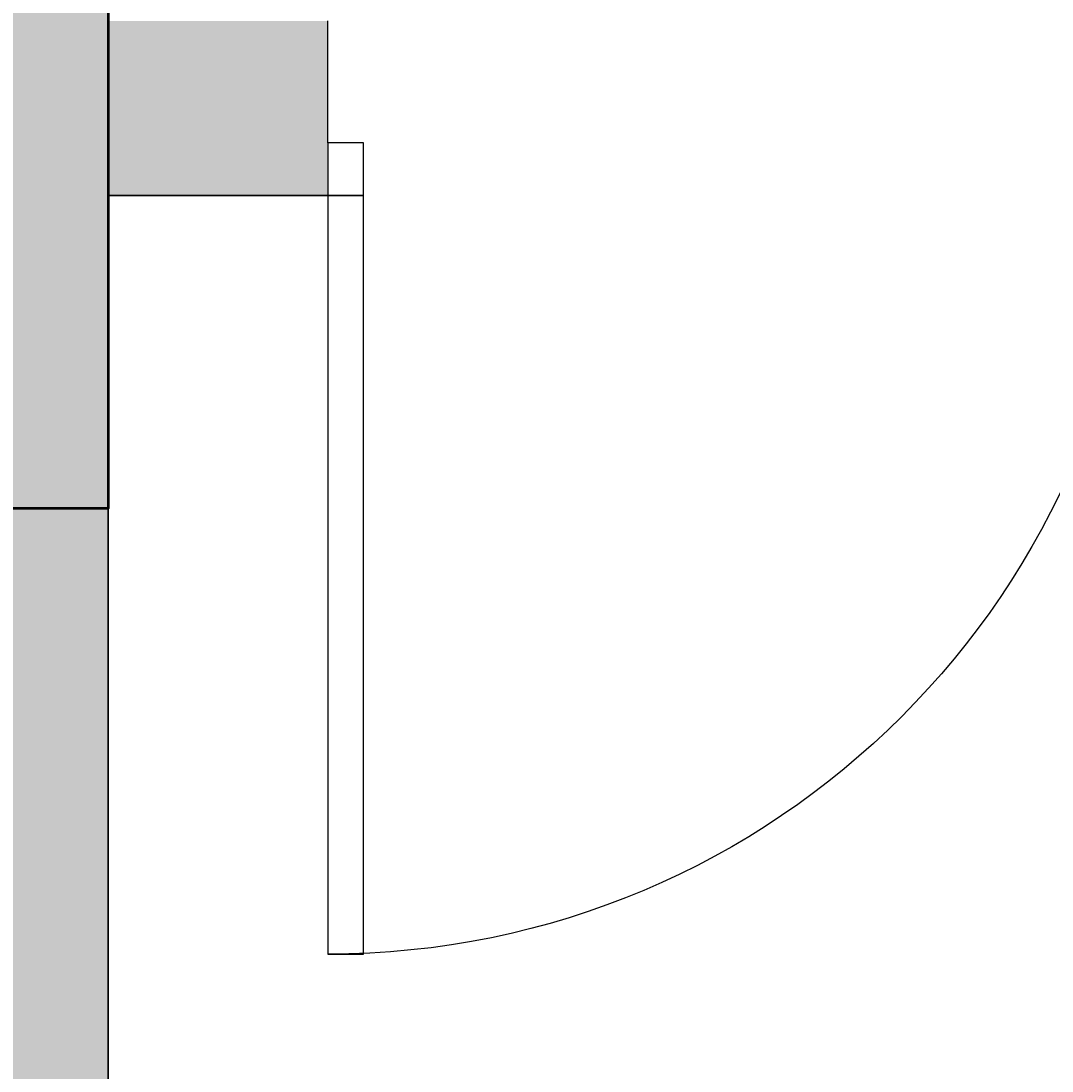
# Model space of a CAD drawing. Units: inches. Extents: x 1998 to 2588, y 1139 to 1977.
# Tile 78 of 134: x 2344 to 2370, y 1454 to 1481. Entities that reach past the tile are written whole.
import ezdxf

# ---------------------------------------------------------------- set-up
doc = ezdxf.new("R2010")
doc.units = ezdxf.units.IN
for name, color, linetype, lineweight in [('A-ANNO-DIMS', 2, 'Continuous', 18), ('A-COLS-PATT', 250, 'Continuous', 13), ('A-WALL-PATT', 252, 'Continuous', 13), ('COLUMN', 10, 'Continuous', 50), ('DOOR', 52, 'Continuous', 25), ('WALL', 200, 'Continuous', 35)]:
    doc.layers.add(name, color=color, linetype=linetype, lineweight=lineweight)
doc.styles.get("Standard").update_dxf_attribs({"font": 'arial.ttf'})
doc.dimstyles.get("Standard").update_dxf_attribs({"dimtxt": 0.18, "dimasz": 0.18, "dimexe": 0.18, "dimexo": 0.0625, "dimgap": 0.09, "dimtad": 0, "dimtih": 1, "dimtoh": 1, "dimdec": 4, "dimzin": 0, "dimdsep": 46, "dimtxsty": 'Standard', "dimcen": 0.09, "dimadec": 0, "dimazin": 0, "dimtfac": 1, "dimtdec": 4, "dimtofl": 0, "dimtmove": 0, "dimatfit": 3, "dimfxl": 1, "dimtolj": 1, "dimtzin": 0, "dimarcsym": 0})

# ---------------------------------------------------------------- blocks, each defined once
blk = doc.blocks.new('*U2')
for p, q in [((0, 0), (0, -6)), ((40, 0), (40, -6))]:
    blk.add_line(p, q)
blk.add_lwpolyline([(0, 0), (0, 40), (1.75, 40), (1.75, 0)], close=True)
blk.add_arc((0, 0), 40, 0, 90)
blk = doc.blocks.new('*D23')
at = {"layer": 'A-ANNO-DIMS', "color": 0, "lineweight": -2, "transparency": 16777216}
for p, q in [((2549.179, 1476.17), (2549.179, 1138.602)), ((2059.473, 1413.17), (2059.473, 1138.602)), ((2059.653, 1138.782), (2303.928, 1138.782)), ((2548.999, 1138.782), (2304.723, 1138.782))]:
    blk.add_line(p, q, dxfattribs=at)
at = {"layer": 'A-ANNO-DIMS', "color": 0, "transparency": 16777216}
for points in [[(2059.653, 1138.812), (2059.653, 1138.752), (2059.473, 1138.782)], [(2548.999, 1138.812), (2548.999, 1138.752), (2549.179, 1138.782)]]:
    blk.add_solid(points, dxfattribs=at)
at = {"layer": 'Defpoints', "color": 0, "transparency": 16777216}
for p in [(2549.179, 1476.232), (2059.473, 1413.232), (2549.179, 1138.782)]:
    blk.add_point(p, dxfattribs=at)
at = {"layer": 'A-ANNO-DIMS', "color": 0, "transparency": 16777216, "insert": (2304.326, 1138.782), "char_height": 0.18, "attachment_point": 5}
blk.add_mtext('\\A1;489.7', dxfattribs=at)
blk = doc.blocks.new('*D43')
at = {"layer": 'A-ANNO-DIMS', "color": 0, "lineweight": -2, "transparency": 16777216}
for p, q in [((2407.973, 1594.67), (2407.973, 1138.602)), ((2345.973, 1588.67), (2345.973, 1138.602)), ((2346.153, 1138.782), (2376.754, 1138.782)), ((2407.793, 1138.782), (2377.191, 1138.782))]:
    blk.add_line(p, q, dxfattribs=at)
at = {"layer": 'A-ANNO-DIMS', "color": 0, "transparency": 16777216}
for points in [[(2346.153, 1138.812), (2346.153, 1138.752), (2345.973, 1138.782)], [(2407.793, 1138.812), (2407.793, 1138.752), (2407.973, 1138.782)]]:
    blk.add_solid(points, dxfattribs=at)
at = {"layer": 'Defpoints', "color": 0, "transparency": 16777216}
for p in [(2407.973, 1594.732), (2345.973, 1588.732), (2407.973, 1138.782)]:
    blk.add_point(p, dxfattribs=at)
at = {"layer": 'A-ANNO-DIMS', "color": 0, "transparency": 16777216, "insert": (2376.973, 1138.782), "char_height": 0.18, "attachment_point": 5}
blk.add_mtext('\\A1;62', dxfattribs=at)

msp = doc.modelspace()

# ---------------------------------------------------------------- hatches: boundary and pattern name
at = {"layer": 'A-COLS-PATT'}
h = msp.add_hatch(color=256, dxfattribs=at)
h.dxf.hatch_style = 1
h.paths.add_polyline_path([(2099.4125, 1888.7324), (2087.9729, 1888.7324), (2087.9729, 1868.3278), (2099.4125, 1868.3278)])
h.paths.add_polyline_path([(2234.4125, 1888.7324), (2222.9729, 1888.7324), (2222.9729, 1868.3278), (2234.4125, 1868.3278)])
h.paths.add_polyline_path([(2341.4729, 1886.637), (2330.0332, 1886.637), (2330.0332, 1866.2324), (2341.4729, 1866.2324)])
h.paths.add_polyline_path([(2507.8006, 1882.7324), (2487.396, 1882.7324), (2487.396, 1871.2927), (2507.8006, 1871.2927)])
h.paths.add_polyline_path([(2510.9729, 1766.672), (2490.5682, 1766.672), (2490.5682, 1755.2324), (2510.9729, 1755.2324)])
h.paths.add_polyline_path([(2345.9729, 1759.7324), (2334.5332, 1759.7324), (2334.5332, 1739.3278), (2345.9729, 1739.3278)])
h.paths.add_polyline_path([(2234.4125, 1774.3318), (2222.9729, 1774.3318), (2222.9729, 1753.9272), (2234.4125, 1753.9272)])
h.paths.add_polyline_path([(2099.4125, 1775.637), (2087.9729, 1775.637), (2087.9729, 1755.2324), (2099.4125, 1755.2324)])
h.paths.add_polyline_path([(2098.0956, 1593.7241), (2077.691, 1593.7241), (2077.691, 1582.2845), (2098.0956, 1582.2845)])
h.paths.add_polyline_path([(2227.4729, 1604.637), (2216.0332, 1604.637), (2216.0332, 1584.2324), (2227.4729, 1584.2324)])
h.paths.add_polyline_path([(2345.9729, 1647.5211), (2334.5332, 1647.5211), (2334.5332, 1627.1165), (2345.9729, 1627.1165)])
h.paths.add_polyline_path([(2522.3775, 1641.2324), (2501.9729, 1641.2324), (2501.9729, 1629.7927), (2522.3775, 1629.7927)])
h.paths.add_polyline_path([(2522.3775, 1480.7324), (2501.9729, 1480.7324), (2501.9729, 1469.2927), (2522.3775, 1469.2927)])
h.paths.add_polyline_path([(2345.9729, 1488.5616), (2334.5332, 1488.5616), (2334.5332, 1468.1569), (2345.9729, 1468.1569)])
h.paths.add_polyline_path([(2234.4125, 1486.137), (2227.4729, 1486.137), (2227.4729, 1465.7324), (2234.4125, 1465.7324)])
h.paths.add_polyline_path([(2227.4729, 1486.137), (2222.9729, 1486.137), (2222.9729, 1465.7324), (2227.4729, 1465.7324)])
h.paths.add_polyline_path([(2108.3775, 1470.2324), (2087.9729, 1470.2324), (2087.9729, 1458.7927), (2108.3775, 1458.7927)])
h.paths.add_polyline_path([(2096.9729, 1365.5012), (2087.9729, 1365.5012), (2087.9729, 1345.0966), (2096.9729, 1345.0966)])
h.paths.add_polyline_path([(2087.9729, 1365.5012), (2085.5332, 1365.5012), (2085.5332, 1345.0966), (2087.9729, 1345.0966)])
h.paths.add_polyline_path([(2234.4125, 1285.137), (2222.9729, 1285.137), (2222.9729, 1264.7324), (2234.4125, 1264.7324)])
h.paths.add_polyline_path([(2345.9729, 1285.137), (2334.5332, 1285.137), (2334.5332, 1264.7324), (2345.9729, 1264.7324)])
h.paths.add_polyline_path([(2503.1458, 1240.172), (2482.7412, 1240.172), (2482.7412, 1228.7324), (2503.1458, 1228.7324)])
h.paths.add_polyline_path([(2510.9729, 1369.172), (2490.5682, 1369.172), (2490.5682, 1357.7324), (2510.9729, 1357.7324)])
at = {"layer": 'A-WALL-PATT'}
h = msp.add_hatch(color=256, dxfattribs=at)
h.dxf.hatch_style = 1
h.paths.add_polyline_path([(2222.9729, 1888.7324), (2099.4125, 1888.7324), (2099.4125, 1879.7324), (2222.9729, 1879.7324)])
h.paths.add_polyline_path([(2096.9729, 1868.3278), (2087.9729, 1868.3278), (2087.9729, 1775.637), (2096.9729, 1775.637)])
h.paths.add_polyline_path([(2227.4729, 1868.3278), (2222.9729, 1868.3278), (2222.9729, 1774.3318), (2227.4729, 1774.3318)])
h.paths.add_polyline_path([(2188.3019, 1759.7324), (2138.6074, 1759.7324), (2099.4125, 1759.7324), (2099.4125, 1755.2324), (2176.9729, 1755.2324), (2188.3019, 1755.2324)])
h.paths.add_polyline_path([(2087.9729, 1759.7324), (2059.4729, 1759.7324), (2059.4729, 1702.7324), (2087.9729, 1702.7324), (2087.9729, 1707.2324), (2063.9729, 1707.2324), (2063.9729, 1755.2324), (2087.9729, 1755.2324)])
h.paths.add_polyline_path([(2096.9729, 1755.2324), (2087.9729, 1755.2324), (2087.9729, 1707.2324), (2096.9729, 1707.2324)])
h.paths.add_polyline_path([(2187.0461, 1707.2324), (2105.9729, 1707.2324), (2096.9729, 1707.2324), (2087.9729, 1707.2324), (2087.9729, 1702.7324), (2105.9729, 1702.7324), (2114.9729, 1702.7324), (2187.0461, 1702.7324)])
h.paths.add_polyline_path([(2181.4729, 1719.2028), (2176.9729, 1719.2028), (2176.9729, 1707.2324), (2181.4729, 1707.2324)])
h.paths.add_polyline_path([(2216.0332, 1588.7324), (2114.9729, 1588.7324), (2105.9729, 1588.7324), (2105.9729, 1584.2324), (2216.0332, 1584.2324)])
h.paths.add_polyline_path([(2077.691, 1588.7324), (2061.4729, 1588.7324), (2061.4729, 1584.2324), (2077.691, 1584.2324)])
h.paths.add_polyline_path([(2105.9729, 1588.7324), (2098.0956, 1588.7324), (2098.0956, 1584.2324), (2105.9729, 1584.2324)])
h.paths.add_polyline_path([(2114.9729, 1596.2642), (2110.1012, 1596.2642), (2105.9729, 1596.2642), (2105.9729, 1588.7324), (2114.9729, 1588.7324)])
h.paths.add_polyline_path([(2114.9729, 1584.2324), (2105.9729, 1584.2324), (2105.9729, 1580.249), (2110.1012, 1580.249), (2114.9729, 1580.249)])
h.paths.add_polyline_path([(2114.9729, 1547.7716), (2110.1012, 1547.7716, -0.0318759), (2105.9729, 1548.035), (2105.9729, 1470.2324), (2108.3775, 1470.2324), (2108.3775, 1465.7324), (2186.2943, 1465.7324), (2186.2943, 1470.2324), (2114.9729, 1470.2324)])
h.paths.add_polyline_path([(2227.4729, 1584.2324), (2222.9729, 1584.2324), (2222.9729, 1486.137), (2227.4729, 1486.137)])
h.paths.add_polyline_path([(2295.4138, 1593.2324), (2227.4729, 1593.2324), (2227.4729, 1588.7324), (2295.4138, 1588.7324), (2295.4138, 1591.8729)])
h.paths.add_polyline_path([(2345.9729, 1627.1165), (2341.4729, 1627.1165), (2341.4729, 1593.2324), (2337.2869, 1593.2324), (2337.2869, 1591.8729), (2337.2869, 1588.7324), (2345.9729, 1588.7324)])
h.paths.add_polyline_path([(2291.9729, 1588.7324), (2287.4729, 1588.7324), (2287.4729, 1522.7324), (2291.9729, 1522.7324)])
h.paths.add_polyline_path([(2291.9729, 1522.7324), (2287.4729, 1522.7324), (2227.4729, 1522.7324), (2227.4729, 1518.2324), (2291.9729, 1518.2324)])
h.paths.add_polyline_path([(2295.7347, 1519.5919), (2295.7347, 1522.7324), (2291.9729, 1522.7324), (2291.9729, 1518.2324), (2295.7347, 1518.2324)])
h.paths.add_polyline_path([(2345.9729, 1522.7324), (2337.6078, 1522.7324), (2337.6078, 1519.5919), (2337.6078, 1518.2324), (2341.4729, 1518.2324), (2341.4729, 1488.5616), (2345.9729, 1488.5616)])
h.paths.add_polyline_path([(2345.9729, 1468.1569), (2341.4729, 1468.1569), (2341.4729, 1374.2324), (2227.4729, 1374.2324), (2227.4729, 1369.7324), (2345.9729, 1369.7324)])
h.paths.add_polyline_path([(2345.9729, 1369.7324), (2341.4729, 1369.7324), (2341.4729, 1362.2324), (2345.9729, 1362.2324)])
h.paths.add_polyline_path([(2345.9729, 1317.7324), (2345.9729, 1322.2324), (2341.4729, 1322.2324), (2341.4729, 1285.137), (2345.9729, 1285.137)], flags=17)
h.paths.add_polyline_path([(2356.2096, 1322.2324), (2345.9729, 1322.2324), (2345.9729, 1317.7324), (2356.2096, 1317.7324), (2356.2096, 1319.3088)], flags=17)
h.paths.add_polyline_path([(2393.9729, 1322.2324), (2375.6999, 1322.2324), (2375.6999, 1319.3088, -0.0202458), (2375.636, 1317.7324), (2393.9729, 1317.7324)], flags=17)
h.paths.add_polyline_path([(2398.4729, 1322.2324), (2393.9729, 1322.2324), (2393.9729, 1317.7324), (2393.9729, 1237.7324), (2345.9729, 1237.7324), (2345.9729, 1264.7324), (2341.4729, 1264.7324), (2341.4729, 1228.7324), (2393.9729, 1228.7324), (2482.7412, 1228.7324), (2482.7412, 1237.7324), (2398.4729, 1237.7324), (2398.4729, 1297.1029)])
h.paths.add_polyline_path([(2398.4729, 1362.2324), (2393.9729, 1362.2324), (2393.9729, 1357.7324), (2398.4729, 1357.7324)])
h.paths.add_polyline_path([(2345.9729, 1329.7549), (2341.4729, 1329.7549), (2341.4729, 1322.2324), (2345.9729, 1322.2324)])
h = msp.add_hatch(color=256, dxfattribs=at)
h.dxf.hatch_style = 1
h.paths.add_polyline_path([(2527.4729, 1362.2324), (2510.9729, 1362.2324), (2510.9729, 1357.7324), (2518.4729, 1357.7324), (2518.4729, 1237.7324), (2503.1458, 1237.7324), (2503.1458, 1228.7324), (2527.4729, 1228.7324)])
h.paths.add_polyline_path([(2490.5682, 1362.2324), (2398.4729, 1362.2324), (2398.4729, 1357.7324), (2490.5682, 1357.7324)])
h.paths.add_polyline_path([(2224.9729, 1264.7324), (2222.9729, 1264.7324), (2222.9729, 1232.4125), (2341.4729, 1232.4125), (2341.4729, 1234.4125), (2224.9729, 1234.4125)])
h.paths.add_polyline_path([(2334.5332, 1273.7324), (2264.7638, 1273.7324), (2264.7638, 1269.5611, -0.043659), (2264.3413, 1264.7324), (2334.5332, 1264.7324)])
h.paths.add_polyline_path([(2236.9551, 1273.7324), (2234.4125, 1273.7324), (2234.4125, 1264.7324), (2236.9551, 1264.7324), (2236.9551, 1269.5611)])
h.paths.add_polyline_path([(2222.9729, 1293.2324), (2096.9729, 1293.2324), (2096.9729, 1345.0966), (2087.9729, 1345.0966), (2087.9729, 1284.2324), (2222.9729, 1284.2324), (2222.9729, 1285.137)])
h.paths.add_polyline_path([(2096.9729, 1458.7927), (2087.9729, 1458.7927), (2087.9729, 1417.7324), (2087.9729, 1413.2324), (2096.9729, 1413.2324), (2096.9729, 1417.7324)])
h.paths.add_polyline_path([(2096.9729, 1413.2324), (2087.9729, 1413.2324), (2087.9729, 1365.5012), (2096.9729, 1365.5012), (2096.9729, 1369.3358)])
h.paths.add_polyline_path([(2186.2943, 1417.7324), (2138.6074, 1417.7324), (2096.9729, 1417.7324), (2096.9729, 1413.2324), (2138.6074, 1413.2324), (2186.2943, 1413.2324)])
h.paths.add_polyline_path([(2181.4729, 1465.7324), (2176.9729, 1465.7324), (2176.9729, 1451.6434), (2181.4729, 1451.6434)])
h.paths.add_polyline_path([(2181.4729, 1422.1664), (2176.9729, 1422.1664), (2176.9729, 1417.7324), (2181.4729, 1417.7324)])
h.paths.add_polyline_path([(2063.9729, 1465.7324), (2087.9729, 1465.7324), (2087.9729, 1470.2324), (2059.4729, 1470.2324), (2059.4729, 1413.2324), (2087.9729, 1413.2324), (2087.9729, 1417.7324), (2063.9729, 1417.7324)])
h.paths.add_polyline_path([(2181.4729, 1755.2324), (2176.9729, 1755.2324), (2176.9729, 1748.6798), (2177.0513, 1748.6798), (2181.4729, 1748.6798)])
h.paths.add_polyline_path([(2227.4729, 1707.2324), (2220.4647, 1707.2324), (2220.4647, 1702.7324), (2222.9729, 1702.7324), (2222.9729, 1604.637), (2227.4729, 1604.637)])
h.paths.add_polyline_path([(2114.9729, 1702.7324), (2105.9729, 1702.7324), (2105.9729, 1628.4781, -0.0318759), (2110.1012, 1628.7416), (2114.9729, 1628.7416)])
h.paths.add_polyline_path([(2345.9729, 1739.3278), (2341.4729, 1739.3278), (2341.4729, 1647.5211), (2345.9729, 1647.5211)])
h.paths.add_polyline_path([(2350.6273, 1641.2324), (2345.9729, 1641.2324), (2345.9729, 1636.7324), (2350.6273, 1636.7324), (2350.6273, 1639.8729)])
h.paths.add_polyline_path([(2501.9729, 1641.2324), (2407.9729, 1641.2324), (2392.5005, 1641.2324), (2392.5005, 1639.8729), (2392.5005, 1636.7324), (2501.9729, 1636.7324)])
h.paths.add_polyline_path([(2510.9729, 1755.2324), (2501.9729, 1755.2324), (2501.9729, 1641.2324), (2510.9729, 1641.2324)])
h.paths.add_polyline_path([(2549.1786, 1641.2324), (2522.3775, 1641.2324), (2522.3775, 1636.7324), (2540.1786, 1636.7324), (2540.1786, 1480.7324), (2522.3775, 1480.7324), (2522.3775, 1476.2324), (2549.1786, 1476.2324)])
h.paths.add_polyline_path([(2498.1786, 1594.7324), (2407.9729, 1594.7324), (2407.9729, 1585.7324), (2416.9729, 1585.7324), (2489.1786, 1585.7324), (2489.1786, 1531.7324), (2416.9729, 1531.7324), (2407.9729, 1531.7324), (2407.9729, 1522.7324), (2498.1786, 1522.7324)])
h.paths.add_polyline_path([(2351.6437, 1480.7324), (2345.9729, 1480.7324), (2345.9729, 1476.2324), (2351.6437, 1476.2324), (2351.6437, 1477.5919)])
h.paths.add_polyline_path([(2501.9729, 1480.7324), (2498.1786, 1480.7324), (2407.9729, 1480.7324), (2393.5168, 1480.7324), (2393.5168, 1477.5919), (2393.5168, 1476.2324), (2501.9729, 1476.2324)])

# ---------------------------------------------------------------- linework, layer by layer
at = {"layer": 'COLUMN'}
msp.add_lwpolyline([(2334.5332, 1488.5616), (2345.9729, 1488.5616), (2345.9729, 1468.1569), (2334.5332, 1468.1569)], close=True, dxfattribs=at)
at = {"layer": 'WALL'}
for p, q in [((2345.9729, 1522.7324), (2345.9729, 1369.7324)), ((2345.9729, 1476.2324), (2352.5596, 1476.2324)), ((2345.9729, 1476.2324), (2352.5596, 1476.2324))]:
    msp.add_line(p, q, dxfattribs=at)

# ---------------------------------------------------------------- block references
at = {"layer": 'DOOR', "xscale": -0.5234138920659225, "yscale": 0.5234138920659225, "zscale": 0.5234138920659225, "rotation": 180}
msp.add_blockref('*U2', (2351.6437, 1477.5919), dxfattribs=at)

# ---------------------------------------------------------------- dimensions: what is measured, and where the dimension line sits
at = {"layer": 'A-ANNO-DIMS'}
for base, p1, p2, override, picture, middle in [((2407.9729, 1138.7824), (2345.9729, 1588.7324), (2407.9729, 1594.7324), {"dimdec": 0, "dimlfac": 1, "dimrnd": 0, "dimzin": 0, "dimdsep": 46, "dimlunit": 2}, '*D43', (2376.9729, 1138.7824)), ((2549.1786, 1138.7824), (2059.4729, 1413.2324), (2549.1786, 1476.2324), {"dimdec": 1, "dimlfac": 1, "dimrnd": 0, "dimzin": 0, "dimdsep": 46, "dimlunit": 2}, '*D23', (2304.3257, 1138.7824))]:
    dim = msp.add_linear_dim(base=base, p1=p1, p2=p2, dimstyle='Standard', override=override, dxfattribs=at)
    dim.commit()
    dim.dimension.update_dxf_attribs({"geometry": picture, "text_midpoint": middle})

doc.saveas('drawing.dxf')
